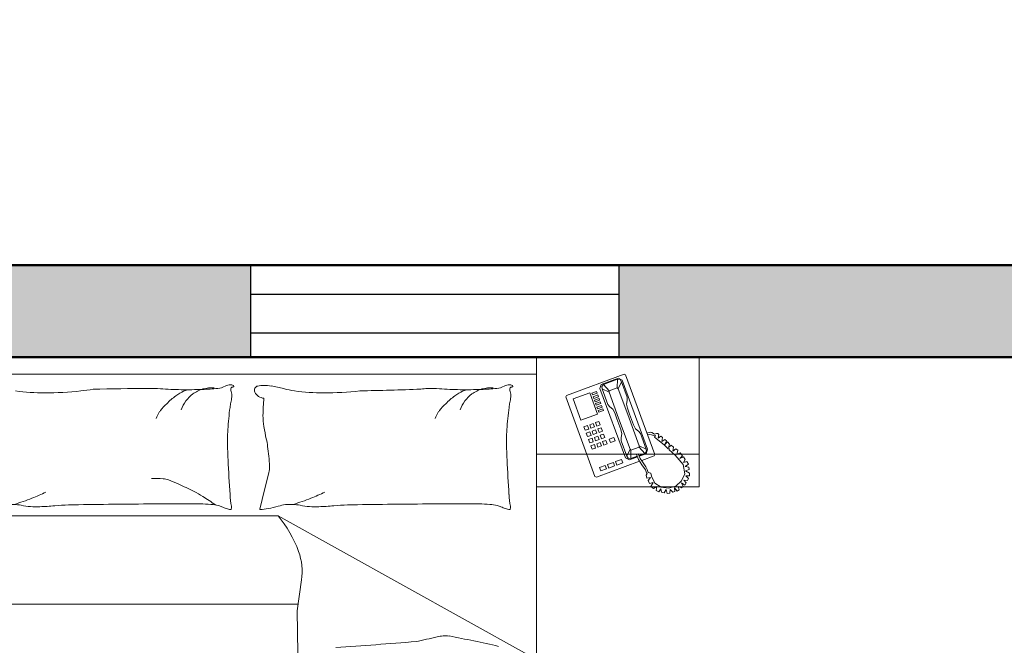
# Model space of a CAD drawing. Units: inches. Extents: x -7 to 1228, y -146 to 1091.
# Tile 55 of 88: x 96 to 193, y 964 to 1025. Entities that reach past the tile are written whole.
import ezdxf

# ---------------------------------------------------------------- set-up
doc = ezdxf.new("R2010")
doc.units = ezdxf.units.IN
for name, color, linetype, lineweight in [('A-FURN', 8, 'Continuous', 18), ('A-GLAZ', 175, 'Continuous', 25), ('A-WALL', 7, 'Continuous', 50), ('A-WALL-PATT', 251, 'Continuous', 13)]:
    doc.layers.add(name, color=color, linetype=linetype, lineweight=lineweight)
doc.styles.add('DIM_FONT', font='SIMPLEX.shx', dxfattribs={"width": 0.8})

# ---------------------------------------------------------------- blocks, each defined once
blk = doc.blocks.new('A$C4F634EDD')
for p, q in [((0.5, 2.6295), (2.3, 2.6295)), ((2.3, 2.6295), (2.3, 0.5295)), ((2.3, 2.6295), (2.8, 2.6295)), ((2.3, 2.2295), (2.3, 2.6295)), ((2.8, 2.6295), (2.8, 2.2295)), ((0.5, 2.5771), (2.3, 2.5771)), ((2.392, 2.5115), (2.5692, 2.5765)), ((2.4985, 2.5445), (2.5516, 2.564)), ((2.5062, 2.5454), (2.5487, 2.561)), ((2.5483, 2.5347), (2.5487, 2.561)), ((2.5487, 2.561), (2.5571, 2.56)), ((2.5615, 2.5536), (2.5514, 2.5318)), ((2.5516, 2.564), (2.5637, 2.5584)), ((2.5571, 2.56), (2.5615, 2.5536)), ((2.5615, 2.5536), (2.5791, 2.5058)), ((2.5637, 2.5584), (2.6418, 2.3458)), ((2.5692, 2.5765), (2.574, 2.5743)), ((2.574, 2.5743), (2.6638, 2.3298)), ((2.412, 2.5007), (2.4634, 2.5196)), ((2.4634, 2.5196), (2.4875, 2.454)), ((2.4842, 2.5232), (2.47, 2.518)), ((2.47, 2.518), (2.472, 2.5127)), ((2.472, 2.5127), (2.4862, 2.5179)), ((2.4862, 2.5179), (2.4842, 2.5232)), ((2.4946, 2.5331), (2.4985, 2.5445)), ((2.5734, 2.3187), (2.4946, 2.5331)), ((2.5062, 2.5454), (2.5004, 2.5392)), ((2.5004, 2.5392), (2.5013, 2.5315)), ((2.5013, 2.5315), (2.5188, 2.4836)), ((2.5013, 2.5315), (2.5231, 2.5214)), ((2.5235, 2.5256), (2.5062, 2.5454)), ((2.5231, 2.5214), (2.5235, 2.5256)), ((2.5523, 2.4417), (2.5231, 2.5214)), ((2.5483, 2.5347), (2.5235, 2.5256)), ((2.5514, 2.5318), (2.5483, 2.5347)), ((2.5807, 2.4521), (2.5514, 2.5318)), ((2.3898, 2.5066), (2.392, 2.5115)), ((2.4795, 2.2621), (2.3898, 2.5066)), ((2.4361, 2.4352), (2.412, 2.5007)), ((2.4881, 2.5126), (2.4739, 2.5074)), ((2.4739, 2.5074), (2.4759, 2.502)), ((2.4759, 2.502), (2.4901, 2.5073)), ((2.492, 2.5019), (2.4778, 2.4967)), ((2.4778, 2.4967), (2.4798, 2.4914)), ((2.4798, 2.4914), (2.494, 2.4966)), ((2.4959, 2.4913), (2.4817, 2.4861)), ((2.4901, 2.5073), (2.4881, 2.5126)), ((2.494, 2.4966), (2.492, 2.5019)), ((2.4979, 2.486), (2.4959, 2.4913)), ((2.5788, 2.4956), (2.5767, 2.4848)), ((2.5791, 2.5058), (2.5788, 2.4956)), ((2.4817, 2.4861), (2.4837, 2.4808)), ((2.4837, 2.4808), (2.4979, 2.486)), ((2.4998, 2.4807), (2.4856, 2.4755)), ((2.4856, 2.4755), (2.4876, 2.4702)), ((2.4876, 2.4702), (2.5018, 2.4754)), ((2.5037, 2.47), (2.4895, 2.4648)), ((2.4895, 2.4648), (2.4915, 2.4595)), ((2.4915, 2.4595), (2.5057, 2.4647)), ((2.5018, 2.4754), (2.4998, 2.4807)), ((2.5057, 2.4647), (2.5037, 2.47)), ((2.5188, 2.4836), (2.5256, 2.4761)), ((2.5256, 2.4761), (2.5342, 2.4692)), ((2.5342, 2.4692), (2.5405, 2.4574)), ((2.5405, 2.4574), (2.547, 2.4397)), ((2.5767, 2.4848), (2.5795, 2.4717)), ((2.5795, 2.4717), (2.586, 2.454)), ((2.4875, 2.454), (2.4361, 2.4352)), ((2.4811, 2.4276), (2.4917, 2.4315)), ((2.485, 2.4169), (2.4811, 2.4276)), ((2.4917, 2.4315), (2.4956, 2.4208)), ((2.5594, 2.4061), (2.547, 2.4397)), ((2.5523, 2.4417), (2.5875, 2.346)), ((2.5807, 2.4521), (2.6158, 2.3564)), ((2.5984, 2.4204), (2.586, 2.454)), ((2.4457, 2.4146), (2.4563, 2.4185)), ((2.4496, 2.4039), (2.4457, 2.4146)), ((2.4602, 2.4078), (2.4496, 2.4039)), ((2.4528, 2.3951), (2.4635, 2.399)), ((2.4563, 2.4185), (2.4602, 2.4078)), ((2.4634, 2.4211), (2.474, 2.425)), ((2.4673, 2.4104), (2.4634, 2.4211)), ((2.4635, 2.399), (2.4674, 2.3883)), ((2.4779, 2.4143), (2.4673, 2.4104)), ((2.4706, 2.4016), (2.4812, 2.4055)), ((2.4745, 2.3909), (2.4706, 2.4016)), ((2.474, 2.425), (2.4779, 2.4143)), ((2.4812, 2.4055), (2.4851, 2.3949)), ((2.4956, 2.4208), (2.485, 2.4169)), ((2.4883, 2.4081), (2.4989, 2.412)), ((2.4922, 2.3975), (2.4883, 2.4081)), ((2.5028, 2.4014), (2.4922, 2.3975)), ((2.4989, 2.412), (2.5028, 2.4014)), ((2.5622, 2.393), (2.5594, 2.4061)), ((2.6047, 2.4086), (2.5984, 2.4204)), ((2.6133, 2.4017), (2.6047, 2.4086)), ((2.6201, 2.3941), (2.6133, 2.4017)), ((2.6499, 2.3979), (2.6397, 2.3953)), ((2.6551, 2.397), (2.6499, 2.3979)), ((2.6627, 2.392), (2.6551, 2.397)), ((2.4567, 2.3844), (2.4528, 2.3951)), ((2.4674, 2.3883), (2.4567, 2.3844)), ((2.46, 2.3756), (2.4706, 2.3795)), ((2.4639, 2.365), (2.46, 2.3756)), ((2.4745, 2.3689), (2.4639, 2.365)), ((2.4706, 2.3795), (2.4745, 2.3689)), ((2.4851, 2.3949), (2.4745, 2.3909)), ((2.4777, 2.3821), (2.4883, 2.386)), ((2.4816, 2.3715), (2.4777, 2.3821)), ((2.4922, 2.3754), (2.4816, 2.3715)), ((2.4849, 2.3626), (2.4955, 2.3665)), ((2.4883, 2.386), (2.4922, 2.3754)), ((2.4954, 2.3886), (2.5061, 2.3925)), ((2.4993, 2.378), (2.4954, 2.3886)), ((2.4955, 2.3665), (2.4994, 2.3559)), ((2.51, 2.3819), (2.4993, 2.378)), ((2.5026, 2.3691), (2.5132, 2.373)), ((2.5065, 2.3585), (2.5026, 2.3691)), ((2.5061, 2.3925), (2.51, 2.3819)), ((2.5132, 2.373), (2.5171, 2.3624)), ((2.5238, 2.3769), (2.538, 2.3821)), ((2.5277, 2.3663), (2.5238, 2.3769)), ((2.5419, 2.3715), (2.5277, 2.3663)), ((2.538, 2.3821), (2.5419, 2.3715)), ((2.5598, 2.372), (2.5601, 2.3822)), ((2.5774, 2.3242), (2.5598, 2.372)), ((2.5601, 2.3822), (2.5622, 2.393)), ((2.6376, 2.3463), (2.6201, 2.3941)), ((2.6417, 2.39), (2.6488, 2.391)), ((2.6488, 2.391), (2.6538, 2.3895)), ((2.6538, 2.3895), (2.6596, 2.388)), ((2.6596, 2.388), (2.6626, 2.3867)), ((2.6626, 2.3867), (2.6662, 2.388)), ((2.6692, 2.394), (2.6627, 2.392)), ((2.6662, 2.388), (2.6632, 2.3828)), ((2.6632, 2.3828), (2.6736, 2.3744)), ((2.6736, 2.3944), (2.6692, 2.394)), ((2.6765, 2.391), (2.6736, 2.3944)), ((2.6736, 2.3744), (2.6922, 2.3593)), ((2.6742, 2.3795), (2.6765, 2.391)), ((2.6824, 2.3858), (2.6742, 2.3795)), ((2.6873, 2.3815), (2.6824, 2.3858)), ((2.6853, 2.369), (2.6873, 2.3815)), ((2.6946, 2.376), (2.6853, 2.369)), ((2.6995, 2.3713), (2.6946, 2.376)), ((2.695, 2.3603), (2.6995, 2.3713)), ((2.7031, 2.3682), (2.695, 2.3603)), ((2.7096, 2.3616), (2.7031, 2.3682)), ((2.4672, 2.3561), (2.4778, 2.36)), ((2.4711, 2.3455), (2.4672, 2.3561)), ((2.4817, 2.3494), (2.4711, 2.3455)), ((2.4778, 2.36), (2.4817, 2.3494)), ((2.4888, 2.352), (2.4849, 2.3626)), ((2.4994, 2.3559), (2.4888, 2.352)), ((2.5171, 2.3624), (2.5065, 2.3585)), ((2.5774, 2.3242), (2.5875, 2.346)), ((2.5875, 2.346), (2.5905, 2.3431)), ((2.5905, 2.3431), (2.5901, 2.3168)), ((2.6154, 2.3522), (2.5905, 2.3431)), ((2.6158, 2.3564), (2.6154, 2.3522)), ((2.6154, 2.3522), (2.6327, 2.3324)), ((2.6376, 2.3463), (2.6158, 2.3564)), ((2.6327, 2.3324), (2.6385, 2.3386)), ((2.6418, 2.3458), (2.6369, 2.332)), ((2.6385, 2.3386), (2.6376, 2.3463)), ((2.6922, 2.3593), (2.7051, 2.3473)), ((2.7051, 2.3473), (2.7079, 2.3475)), ((2.7062, 2.351), (2.7096, 2.3616)), ((2.7147, 2.3578), (2.7062, 2.351)), ((2.7079, 2.3475), (2.7079, 2.3443)), ((2.7079, 2.3443), (2.727, 2.3277)), ((2.7214, 2.3517), (2.7147, 2.3578)), ((2.7196, 2.34), (2.7214, 2.3517)), ((2.7286, 2.3466), (2.7196, 2.34)), ((2.7346, 2.3423), (2.7286, 2.3466)), ((2.732, 2.3295), (2.7346, 2.3423)), ((2.8, 2.3301), (2.3, 2.3301)), ((2.6172, 2.3086), (2.4844, 2.2599)), ((2.5362, 2.305), (2.5185, 2.2985)), ((2.5401, 2.2944), (2.5362, 2.305)), ((2.561, 2.3141), (2.5433, 2.3076)), ((2.5433, 2.3076), (2.5472, 2.297)), ((2.5649, 2.3035), (2.561, 2.3141)), ((2.5855, 2.3131), (2.5734, 2.3187)), ((2.5818, 2.3178), (2.5774, 2.3242)), ((2.5901, 2.3168), (2.5818, 2.3178)), ((2.6104, 2.3222), (2.5855, 2.3131)), ((2.5901, 2.3168), (2.6097, 2.324)), ((2.613, 2.3312), (2.6077, 2.3293)), ((2.6077, 2.3293), (2.6135, 2.3141)), ((2.6192, 2.3174), (2.613, 2.3312)), ((2.6135, 2.3141), (2.6244, 2.2977)), ((2.6153, 2.3261), (2.6327, 2.3324)), ((2.6369, 2.332), (2.6161, 2.3243)), ((2.626, 2.3069), (2.6192, 2.3174)), ((2.6616, 2.3249), (2.6234, 2.3109)), ((2.6365, 2.2916), (2.626, 2.3069)), ((2.6638, 2.3298), (2.6616, 2.3249)), ((2.727, 2.3277), (2.7512, 2.2983)), ((2.7423, 2.3345), (2.732, 2.3295)), ((2.7406, 2.3172), (2.7495, 2.325)), ((2.7519, 2.3218), (2.7406, 2.3172)), ((2.7495, 2.325), (2.7423, 2.3345)), ((2.7575, 2.3144), (2.7519, 2.3218)), ((2.7526, 2.3045), (2.7575, 2.3144)), ((2.7622, 2.308), (2.7526, 2.3045)), ((2.7673, 2.2997), (2.7622, 2.308)), ((2.5114, 2.2959), (2.4936, 2.2894)), ((2.4936, 2.2894), (2.4976, 2.2788)), ((2.4976, 2.2788), (2.5153, 2.2853)), ((2.5153, 2.2853), (2.5114, 2.2959)), ((2.5185, 2.2985), (2.5224, 2.2879)), ((2.5224, 2.2879), (2.5401, 2.2944)), ((2.5472, 2.297), (2.5649, 2.3035)), ((2.6244, 2.2977), (2.6349, 2.2825)), ((2.6349, 2.2825), (2.638, 2.273)), ((2.6407, 2.2834), (2.6365, 2.2916)), ((2.6438, 2.2739), (2.6407, 2.2834)), ((2.7512, 2.2983), (2.756, 2.2695)), ((2.7574, 2.2924), (2.7673, 2.2997)), ((2.7687, 2.2905), (2.7574, 2.2924)), ((2.7587, 2.279), (2.7699, 2.2828)), ((2.7708, 2.2725), (2.7587, 2.279)), ((2.7699, 2.2828), (2.7687, 2.2905)), ((1.4546, 2.1912), (1.4752, 2.2738)), ((2.4844, 2.2599), (2.4795, 2.2621)), ((2.6399, 2.2712), (2.6374, 2.2659)), ((2.6374, 2.2659), (2.6398, 2.257)), ((2.638, 2.273), (2.6399, 2.2712)), ((2.6398, 2.257), (2.6509, 2.259)), ((2.6509, 2.259), (2.6431, 2.2492)), ((2.6431, 2.2492), (2.6473, 2.2398)), ((2.6519, 2.2716), (2.6438, 2.2739)), ((2.6535, 2.2628), (2.6519, 2.2716)), ((2.6636, 2.2409), (2.6535, 2.2628)), ((2.7459, 2.2483), (2.7284, 2.2317)), ((2.756, 2.2695), (2.7459, 2.2483)), ((2.7529, 2.2505), (2.7645, 2.2498)), ((2.7607, 2.2424), (2.7529, 2.2505)), ((2.759, 2.2637), (2.7706, 2.2643)), ((2.7676, 2.2559), (2.759, 2.2637)), ((2.7645, 2.2498), (2.7676, 2.2559)), ((2.7706, 2.2643), (2.7708, 2.2725)), ((2.8, 2.2295), (2.3, 2.2295)), ((2.6473, 2.2398), (2.6592, 2.2429)), ((2.6592, 2.2429), (2.6521, 2.2314)), ((2.6521, 2.2314), (2.6598, 2.2248)), ((2.6598, 2.2248), (2.6697, 2.2309)), ((2.6836, 2.2287), (2.6636, 2.2409)), ((2.6697, 2.2309), (2.6684, 2.219)), ((2.6684, 2.219), (2.6761, 2.2145)), ((2.6761, 2.2145), (2.6821, 2.2237)), ((2.6821, 2.2237), (2.6843, 2.2135)), ((2.7063, 2.2256), (2.6836, 2.2287)), ((2.6927, 2.2117), (2.6986, 2.222)), ((2.6986, 2.222), (2.7019, 2.2098)), ((2.7284, 2.2317), (2.7063, 2.2256)), ((2.7102, 2.2104), (2.7113, 2.2218)), ((2.7113, 2.2218), (2.7192, 2.2137)), ((2.7192, 2.2137), (2.7255, 2.2152)), ((2.7255, 2.2152), (2.7242, 2.2265)), ((2.7242, 2.2265), (2.7324, 2.2165)), ((2.7324, 2.2165), (2.7386, 2.2208)), ((2.7386, 2.2208), (2.7354, 2.2306)), ((2.7354, 2.2306), (2.7462, 2.2264)), ((2.7509, 2.2314), (2.7459, 2.2418)), ((2.7459, 2.2418), (2.7568, 2.2352)), ((2.7462, 2.2264), (2.7509, 2.2314)), ((2.7568, 2.2352), (2.7607, 2.2424)), ((1.4471, 2.1612), (1.4546, 2.1912)), ((2.6843, 2.2135), (2.6927, 2.2117)), ((2.7019, 2.2098), (2.7102, 2.2104)), ((1.5035, 2.141), (0.5458, 2.141)), ((1.5035, 2.141), (2.2716, 1.7136)), ((1.576, 1.9433), (1.5624, 1.8479)), ((0.5458, 1.8684), (1.5653, 1.8684)), ((1.5624, 1.8479), (1.5641, 1.7178))]:
    blk.add_line(p, q)
for centre, radius, start, end in [((0.7851, 3.2019), 0.6827, 262.4531, 270), ((0.7851, 3.5682), 1.049, 270, 276.0867), ((0.8402, 3.0514), 0.5293, 276.0867, 280.1899), ((1.1602, -8.1346), 10.6675, 90.30153, 91.21582), ((1.1169, 2.2433), 0.2897, 85.1982, 92.5386), ((1.2142, 3.4021), 0.8732, 265.1982, 269.4243), ((1.2362, 2.45), 0.0768, 117.2396, 128.3886), ((1.3082, 2.3102), 0.234, 110.8603, 117.2396), ((1.2204, 4.0232), 1.4943, 269.4243, 271.9079), ((1.2995, 2.4357), 0.0992, 105.9352, 126.0864), ((1.2429, 3.3501), 0.8208, 271.9079, 275.2592), ((1.2995, 2.4357), 0.0992, 85.7841, 105.9352), ((1.3132, 2.5864), 0.0539, 275.2592, 300.6513), ((1.3554, 2.5152), 0.0289, 85.6975, 120.6513), ((1.3556, 2.519), 0.0251, 68.2117, 85.6975), ((1.3739, 2.5288), 0.0156, 158.0096, 201.421), ((1.3634, 2.533), 0.00428, 78.1069, 158.0096), ((1.3288, 2.5111), 0.0328, 351.8665, 21.421), ((1.3647, 2.5395), 0.00232, 258.1069, 19.564), ((1.3637, 2.5391), 0.00342, 19.564, 68.2117), ((1.444, 2.5274), 0.0131, 101.2724, 206.5805), ((1.4628, 2.5368), 0.0342, 206.5805, 265.5998), ((1.4591, 2.4516), 0.0904, 90, 101.2724), ((1.4591, 2.3808), 0.1611, 81.5628, 90), ((1.438, 2.2388), 0.3048, 74.256, 81.5628), ((1.5865, 2.7653), 0.2422, 254.256, 262.4531), ((1.6443, 3.2019), 0.6827, 262.4531, 270), ((1.6443, 3.5682), 1.049, 270, 276.0867), ((1.4785, 15.4878), 12.9656, 271.22425, 272.05324), ((1.97, 2.3805), 0.1524, 92.5386, 100.1899), ((1.9761, 2.2433), 0.2897, 85.1982, 92.5386), ((2.0734, 3.4021), 0.8732, 265.1982, 269.4243), ((2.0954, 2.45), 0.0768, 117.2396, 128.3886), ((2.1674, 2.3102), 0.234, 110.8603, 117.2396), ((2.0797, 4.0232), 1.4943, 269.4243, 271.9079), ((2.1588, 2.4357), 0.0992, 105.9352, 126.0864), ((2.1021, 3.3501), 0.8208, 271.9079, 275.2592), ((2.1588, 2.4357), 0.0992, 85.7841, 105.9352), ((2.1724, 2.5864), 0.0539, 275.2592, 300.6513), ((2.2146, 2.5152), 0.0289, 85.6975, 120.6513), ((2.2149, 2.519), 0.0251, 68.2117, 85.6975), ((2.2331, 2.5288), 0.0156, 158.0096, 201.421), ((2.2226, 2.533), 0.00428, 78.1069, 158.0096), ((2.1881, 2.5111), 0.0328, 351.8665, 21.421), ((2.224, 2.5395), 0.00232, 258.1069, 19.564), ((2.2229, 2.5391), 0.00342, 19.564, 68.2117), ((1.4317, 2.2032), 0.3916, 128.3886, 133.8115), ((1.2995, 2.4357), 0.0992, 143.8234, 161.5603), ((1.2995, 2.4357), 0.0992, 126.0864, 143.8234), ((1.5522, 2.448), 0.1983, 167.8905, 172.3191), ((1.1177, 2.5413), 0.246, 347.8905, 351.8665), ((1.949, 2.4496), 0.4918, 173.7676, 180), ((2.291, 2.2032), 0.3916, 128.3886, 133.8115), ((2.1588, 2.4357), 0.0992, 143.8234, 161.5603), ((2.1588, 2.4357), 0.0992, 126.0864, 143.8234), ((2.4114, 2.448), 0.1983, 167.8905, 172.3191), ((1.977, 2.5413), 0.246, 347.8905, 351.8665), ((1.3127, 2.3625), 0.2002, 151.6832, 156.9972), ((1.1799, 2.4341), 0.0493, 140.9651, 151.6832), ((1.3165, 2.3233), 0.2252, 133.8115, 140.9651), ((2.2605, 2.3525), 0.9131, 172.3191, 176.6313), ((2.1719, 2.3625), 0.2002, 151.6832, 156.9972), ((2.0391, 2.4341), 0.0493, 140.9651, 151.6832), ((2.1757, 2.3233), 0.2252, 133.8115, 140.9651), ((3.1198, 2.3525), 0.9131, 172.3191, 176.6313), ((1.6611, 2.4496), 0.204, 180, 189.6844), ((2.0266, 2.3663), 0.6787, 176.6313, 181.6331), ((2.3295, 2.5637), 0.882, 189.6844, 192.1984), ((2.8858, 2.3663), 0.6787, 176.6313, 181.6331), ((1.1575, 2.3103), 0.3171, 8.0051, 12.1984), ((2.7128, 2.3859), 1.3652, 181.6331, 183.055), ((0.8191, 2.2627), 0.6588, 2.6649, 8.0051), ((3.5721, 2.3859), 1.3652, 181.6331, 183.055), ((14.9657, 3.0398), 13.6356, 183.05496, 183.50486), ((15.8249, 3.0398), 13.6356, 183.05496, 183.50486), ((1.4096, 2.2902), 0.0677, 345.9548, 2.6649), ((1.1303, 1.9835), 0.2721, 85.9172, 93.5552), ((1.1455, 2.197), 0.058, 69.3257, 85.9172), ((0.9871, 1.7772), 0.5066, 65.6735, 69.3257), ((0.473, 2.8815), 0.7387, 293.4844, 295.3111), ((0.6058, 0.9338), 1.4323, 63.5015, 65.6735), ((1.1054, 1.9358), 0.3126, 57.865, 63.5015), ((1.3322, 2.8815), 0.7387, 293.4844, 295.3111), ((0.473, 2.8815), 0.7387, 287.1982, 289.428), ((0.473, 2.8815), 0.7387, 289.428, 291.6577), ((0.473, 2.8815), 0.7387, 291.6577, 293.4844), ((0.8841, 1.5835), 0.7286, 54.1737, 57.865), ((1.6762, 2.2258), 0.3212, 183.5049, 189.9984), ((1.3322, 2.8815), 0.7387, 287.1982, 289.428), ((1.3322, 2.8815), 0.7387, 289.428, 291.6577), ((1.3322, 2.8815), 0.7387, 291.6577, 293.4844), ((2.5355, 2.2258), 0.3212, 183.5049, 189.9984), ((0.6836, 2.0301), 0.1459, 78.4414, 96.4341), ((0.759, 2.3985), 0.2301, 258.4414, 272.7491), ((0.7026, 3.5718), 1.4048, 272.7491, 274.6176), ((0.9136, 0.9591), 1.2165, 92.6096, 94.6176), ((1.2501, -19.8405), 22.0183, 90.37908, 91.01965), ((1.2012, -3.5404), 5.7185, 89.7135, 90.9704), ((1.224, 1.0141), 1.164, 86.426, 89.7135), ((1.2875, 2.0302), 0.1459, 77.131, 86.426), ((1.3099, 2.1283), 0.0453, 62.7159, 77.131), ((1.3658, 2.2367), 0.0767, 242.7159, 253.7788), ((1.3688, 2.247), 0.0875, 253.7788, 262.8796), ((1.3581, 2.1615), 0.00132, 262.8796, 343.3022), ((1.3409, 2.1667), 0.0193, 343.3022, 9.9984), ((1.448, 2.1609), 0.000917, 165.9551, 274.0829), ((1.4288, 2.4301), 0.2708, 274.0829, 279.4841), ((1.4355, 2.3896), 0.2297, 279.4841, 287.3864), ((1.5399, 2.0561), 0.1197, 96.4341, 107.3864), ((1.5429, 2.0301), 0.1459, 78.4414, 96.4341), ((1.6182, 2.3985), 0.2301, 258.4414, 272.7491), ((1.5619, 3.5718), 1.4048, 272.7491, 274.6176), ((1.7729, 0.9591), 1.2165, 92.6096, 94.6176), ((2.1093, -19.8405), 22.0183, 90.37908, 91.01965), ((2.0605, -3.5404), 5.7185, 89.7135, 90.9704), ((2.0833, 1.0141), 1.164, 86.426, 89.7135), ((2.1467, 2.0302), 0.1459, 77.131, 86.426), ((2.1691, 2.1283), 0.0453, 62.7159, 77.131), ((2.2251, 2.2367), 0.0767, 242.7159, 253.7788), ((2.2281, 2.247), 0.0875, 253.7788, 262.8796), ((2.2174, 2.1615), 0.00132, 262.8796, 343.3022), ((2.2001, 2.1667), 0.0193, 343.3022, 9.9984), ((1.2147, 1.9017), 0.3751, 20.1488, 39.6445), ((1.3977, 1.9688), 0.1801, 351.8644, 20.1488), ((1.4194, 4.2174), 2.5158, 281.6741, 283.1904), ((2.0378, 1.5789), 0.1942, 97.7304, 103.1904), ((2.0195, 1.7137), 0.0581, 79.2724, 97.7304), ((1.2737, -2.2227), 4.0646, 77.0745, 79.2724), ((0.6102, 18.0525), 16.3521, 273.75703, 274.62393)]:
    blk.add_arc(centre, radius, start, end)
at = {"style": 'DIM_FONT', "width": 0.8, "flags": 9}
for tag, p in [('YSIZE', (0.5, 2.6295)), ('XSIZE', (0.5, 2.6295)), ('XSIZE', (2.2985, 2.6295)), ('YSIZE', (2.2985, 2.6295))]:
    blk.add_attdef(tag, p, '', height=0.0005, dxfattribs=at)
blk = doc.blocks.new('WIN-36')
for p, q in [((0, 36), (0, 0)), ((9, 36), (0, 36)), ((2.343, 36), (2.343, 0)), ((6.137, 0), (6.137, 36)), ((9, 0), (9, 36)), ((0, 0), (9, 0)), ((2.343, 0), (6.137, 0))]:
    blk.add_line(p, q)

msp = doc.modelspace()

# ---------------------------------------------------------------- hatches: boundary and pattern name
at = {"layer": 'A-WALL-PATT'}
h = msp.add_hatch(color=256, dxfattribs=at)
h.dxf.hatch_style = 1
h.paths.add_polyline_path([(69, 568), (60, 568), (60, 493), (63.289, 493), (69, 493)])
h.paths.add_polyline_path([(69, 662.405), (60, 662.405), (60, 586), (69, 586)], flags=17)
h.paths.add_polyline_path([(69, 723), (184, 723), (184, 734), (179, 734), (179, 728), (69, 728), (69, 741.623), (60, 741.623), (60, 698.405), (69, 698.405)], flags=17)
h.paths.add_polyline_path([(69, 782), (231, 782), (231, 728), (231, 723), (231, 586), (236, 586), (236, 787), (69, 787), (69, 800.126), (60, 800.126), (60, 765.623), (69, 765.623)])
h.paths.add_polyline_path([(184, 842), (189, 842), (189, 848), (173, 848), (173, 842), (179, 842), (179, 787), (184, 787)])
h.paths.add_polyline_path([(118.22, 69), (69, 69), (69, 60), (118.22, 60)])
h.paths.add_polyline_path([(227, 69), (154.22, 69), (154.22, 60), (227, 60)])
h.paths.add_polyline_path([(236, 60), (232.711, 60), (227, 60), (227, 36), (236, 36)])
h.paths.add_polyline_path([(389, 60), (380, 60), (380, 36), (389, 36)])
h.paths.add_polyline_path([(384, 181), (380, 181), (380, 115), (380, 78), (384, 78)])
h.paths.add_polyline_path([(380, 115), (334.547, 115), (334.547, 109), (380, 109)])
h.paths.add_polyline_path([(274.547, 115), (236, 115), (236, 201), (232.711, 201), (231, 201), (231, 78), (236, 78), (236, 109), (274.547, 109)])
h.paths.add_polyline_path([(69, 123), (60, 123), (60, 78), (69, 78)])
h.paths.add_polyline_path([(69, 201), (60, 201), (60, 159), (69, 159)])
h.paths.add_polyline_path([(143, 219), (69, 219), (69, 213), (143, 213)], flags=17)
h.paths.add_polyline_path([(189, 219), (184, 219), (184, 274), (231, 274), (231, 219), (236, 219), (236, 279), (184, 279), (184, 297), (179, 297), (179, 279), (69, 279), (69, 290.912), (60, 290.912), (60, 262.179), (69, 262.179), (69, 274), (179, 274), (179, 219), (173, 219), (173, 213), (189, 213)])
h.paths.add_polyline_path([(69, 238.179), (60, 238.179), (60, 219), (69, 219)], flags=17)
h.paths.add_polyline_path([(69, 333), (60, 333), (60, 314.912), (69, 314.912), (69, 316.965)])
h.paths.add_polyline_path([(190, 338), (184, 338), (69, 338), (69, 333), (179, 333), (179, 327), (184, 327), (184, 333.021), (190, 333.046)])
h.paths.add_polyline_path([(69, 386.806), (60, 386.806), (60, 351), (69, 351)])
h.paths.add_polyline_path([(69, 475), (60, 475), (60, 422.806), (69, 422.806)])
h.paths.add_polyline_path([(236, 475), (231, 475), (231, 351.238), (236, 351.238)])
h.paths.add_polyline_path([(384, 475), (380, 475), (380, 362), (384, 362)])
h.paths.add_polyline_path([(547, 307), (439, 307), (439, 356), (445, 356), (445, 362), (433, 362), (433, 307), (380, 307), (380, 244), (380, 241), (384, 241), (384, 301), (433, 301), (433, 277), (439, 277), (439, 301), (547, 301)])
h.paths.add_polyline_path([(547, 241), (439, 241), (439, 247), (433, 247), (433, 235), (547, 235)])
h.paths.add_polyline_path([(450, 69), (440.286, 69), (424.889, 69), (389, 69), (389, 60), (450, 60)])
h.paths.add_polyline_path([(547, 69), (486, 69), (486, 60), (547, 60)])
h.paths.add_polyline_path([(556, 148.268), (547, 148.268), (547, 78), (556, 78)])
h.paths.add_polyline_path([(556, 223), (547, 223), (547, 195), (547, 184.268), (556, 184.268)])
h.paths.add_polyline_path([(556, 311.192), (547, 311.192), (547, 273.075), (556, 273.075)])
h.paths.add_polyline_path([(556, 344), (552.711, 344), (547, 344), (547, 335.192), (556, 335.192)])
h.paths.add_polyline_path([(556, 249.075), (547, 249.075), (547, 241), (556, 241)])
h.paths.add_polyline_path([(547, 362), (475, 362), (475, 356), (547, 356)], flags=0)
h.paths.add_polyline_path([(556, 399.621), (547, 399.621), (547, 362), (556, 362)])
h.paths.add_polyline_path([(556, 475), (547, 475), (547, 435.621), (556, 435.621)])
h.paths.add_polyline_path([(547, 493), (389, 493), (389, 487), (547, 487)])
h.paths.add_polyline_path([(380, 493), (278, 493), (278, 487), (380, 487)])
h.paths.add_polyline_path([(227, 493), (69, 493), (69, 487), (227, 487)])
h.paths.add_polyline_path([(643, 122.445), (634, 122.445), (634, 78), (643, 78)])
h.paths.add_polyline_path([(702.5, 69), (692.786, 69), (677.389, 69), (643, 69), (643, 60), (702.5, 60)])
h.paths.add_polyline_path([(798, 69), (738.5, 69), (738.5, 60), (798, 60)])
h.paths.add_polyline_path([(807, 60), (803.711, 60), (798, 60), (798, 36), (807, 36)])
h.paths.add_polyline_path([(807, 109), (846.751, 109), (846.751, 115), (807, 115), (807, 159), (802, 159), (802, 78), (807, 78)])
h.paths.add_polyline_path([(807, 201), (802, 201), (802, 195), (807, 195)])
h.paths.add_polyline_path([(643, 201), (634, 201), (634, 158.445), (643, 158.445)])
h.paths.add_polyline_path([(756, 225), (751, 225), (751, 219), (643, 219), (643, 213), (756, 213)])
h.paths.add_polyline_path([(643, 240.848), (634, 240.848), (634, 219), (643, 219)])
h.paths.add_polyline_path([(643, 274), (643, 288.629), (634, 288.629), (634, 264.848), (643, 264.848)])
h.paths.add_polyline_path([(802, 279), (756, 279), (756, 297), (751, 297), (751, 279), (643, 279), (643, 274), (751, 274), (751, 255), (756, 255), (756, 274), (802, 274)])
h.paths.add_polyline_path([(807, 333), (803.711, 333), (802, 333), (802, 279), (802, 274), (802, 219), (807, 219)])
h.paths.add_polyline_path([(956, 182), (951, 182), (951, 115), (906.751, 115), (906.751, 109), (951, 109), (951, 78), (956, 78)])
h.paths.add_polyline_path([(960, 60), (951, 60), (951, 36), (960, 36)])
h.paths.add_polyline_path([(1021, 69), (1005.781, 69), (960, 69), (960, 60), (1021, 60)])
h.paths.add_polyline_path([(956, 224), (951, 224), (951, 218), (956, 218)])
h.paths.add_polyline_path([(956, 302), (1004, 302), (1004, 278), (1010, 278), (1010, 302), (1118, 302), (1118, 290.809), (1127, 290.809), (1127, 326.968), (1118, 326.968), (1118, 320.966), (1118, 307), (1010, 307), (1010, 356), (1016, 356), (1016, 362), (1004, 362), (1004, 307), (951, 307), (951, 244), (951, 242), (954.289, 242), (956, 242)])
h.paths.add_polyline_path([(643, 333), (634, 333), (634, 312.629), (643, 312.629), (643, 316.965)])
h.paths.add_polyline_path([(756, 338), (643, 338), (643, 333), (751, 333), (751, 327), (756, 327)])
h.paths.add_polyline_path([(643, 388), (634, 388), (634, 351), (643, 351)])
h.paths.add_polyline_path([(807, 357), (802, 357), (802, 351), (807, 351)])
h.paths.add_polyline_path([(807, 475), (802, 475), (802, 393), (807, 393)])
h.paths.add_polyline_path([(643, 475), (634, 475), (634, 424), (643, 424)])
h.paths.add_polyline_path([(798, 493), (643, 493), (643, 487), (798, 487)])
h.paths.add_polyline_path([(634, 493), (556, 493), (556, 487), (634, 487)])
h.paths.add_polyline_path([(813, 493), (807, 493), (807, 487), (813, 487)])
h.paths.add_polyline_path([(951, 493), (849, 493), (849, 487), (951, 487)])
h.paths.add_polyline_path([(956, 484), (951, 484), (951, 374), (956, 374)])
h.paths.add_polyline_path([(1109, 493), (969, 493), (969, 487), (1109, 487)])
h.paths.add_polyline_path([(1127, 484), (1118, 484), (1118, 450.641), (1127, 450.641)])
h.paths.add_polyline_path([(1127, 414.641), (1118, 414.641), (1118, 365), (1127, 365)])
h.paths.add_polyline_path([(1109, 362), (1046, 362), (1046, 356), (1109, 356)], flags=17)
h.paths.add_polyline_path([(1127, 356), (1123.454, 356), (1118, 356), (1118, 350.968), (1127, 350.968)], flags=0)
h.paths.add_polyline_path([(1127, 266.809), (1118, 266.809), (1118, 262.361), (1118, 242), (1127, 242)], flags=17)
h.paths.add_polyline_path([(1118, 242), (1010, 242), (1010, 248), (1004, 248), (1004, 237), (1118, 237)])
h.paths.add_polyline_path([(1127, 224), (1118, 224), (1118, 170), (1127, 170)])
h.paths.add_polyline_path([(1127, 134), (1118, 134), (1118, 78), (1127, 78)])
h.paths.add_polyline_path([(1118, 69), (1057, 69), (1057, 60), (1118, 60)])
h.paths.add_polyline_path([(227, 571.546), (227, 574), (69, 574), (69, 568), (227, 568)])
h.paths.add_polyline_path([(380, 571.546), (380, 574), (278, 574), (278, 568), (380, 568)])
h.paths.add_polyline_path([(242, 574), (236, 574), (236, 568), (242, 568)])
h.paths.add_polyline_path([(547, 571.546), (547, 574), (389, 574), (389, 568), (547, 568)])
h.paths.add_polyline_path([(384, 733), (380, 733), (380, 586), (384, 586)])
h.paths.add_polyline_path([(556, 646), (634, 646), (634, 655), (547, 655), (547, 586), (556, 586)])
h.paths.add_polyline_path([(634, 574), (556, 574), (556, 568), (634, 568)])
h.paths.add_polyline_path([(643, 655), (634, 655), (634, 586), (643, 586)])
h.paths.add_polyline_path([(798, 574), (643, 574), (643, 568), (798, 568)])
h.paths.add_polyline_path([(643, 663.854), (634, 663.854), (634, 655), (643, 655)])
h.paths.add_polyline_path([(556, 676.967), (547, 676.967), (547, 655), (556, 655)])
h.paths.add_polyline_path([(556, 733), (547, 733), (547, 712.967), (556, 712.967)])
h.paths.add_polyline_path([(643, 710), (634, 710), (634, 699.854), (643, 699.854)])
h.paths.add_polyline_path([(807, 668), (802, 668), (802, 586), (807, 586)])
h.paths.add_polyline_path([(951, 574), (849, 574), (849, 568), (951, 568)])
h.paths.add_polyline_path([(956, 691), (951, 691), (951, 577), (956, 577)])
h.paths.add_polyline_path([(1109, 574), (969, 574), (969, 568), (1109, 568)])
h.paths.add_polyline_path([(1127, 643.403), (1118, 643.403), (1118, 577), (1127, 577)])
h.paths.add_polyline_path([(1127, 568), (1123.454, 568), (1118, 568), (1118, 493), (1127, 493)])
h.paths.add_polyline_path([(1127, 733), (1118, 733), (1118, 679.403), (1127, 679.403)])
h.paths.add_polyline_path([(1127, 777.348), (1118, 777.348), (1118, 770.035), (1118, 751), (1127, 751)], flags=17)
h.paths.add_polyline_path([(1118, 751), (1010, 751), (1010, 757), (1004, 757), (1004, 745), (1118, 745)])
h.paths.add_polyline_path([(956, 811), (1004, 811), (1004, 787), (1010, 787), (1010, 811), (1017.874, 811), (1017.874, 811.627, -0.414214), (1018.247, 812), (1031.978, 812, -0.414214), (1032.351, 811.627), (1032.351, 811), (1118, 811), (1118, 801.348), (1127, 801.348), (1127, 834.685), (1118, 834.685), (1118, 830.238), (1118, 817), (1010, 817), (1010, 866), (1016, 866), (1016, 872), (1004, 872), (1004, 817), (956, 817), (956, 866), (951, 866), (951, 751), (954.289, 751), (956, 751)])
h.paths.add_polyline_path([(1118, 872), (1046, 872), (1046, 866), (1118, 866)], flags=17)
h.paths.add_polyline_path([(1127, 924.711), (1118, 924.711), (1118, 884), (1127, 884)])
h.paths.add_polyline_path([(1127, 866), (1123.711, 866), (1118, 866), (1118, 858.685), (1127, 858.685)], flags=17)
h.paths.add_polyline_path([(956, 983), (951, 983), (951, 952), (807, 952), (807, 983), (802, 983), (802, 902), (807, 902), (807, 946), (951, 946), (951, 884), (956, 884)])
h.paths.add_polyline_path([(807, 842), (802, 842), (802, 787), (756, 787), (756, 806), (751, 806), (751, 787), (643, 787), (643, 782), (751, 782), (751, 764), (756, 764), (756, 782), (802, 782), (802, 728), (807, 728)])
h.paths.add_polyline_path([(756, 848), (643, 848), (643, 842), (751, 842), (751, 836), (756, 836)])
h.paths.add_polyline_path([(756, 734), (751, 734), (751, 728), (643, 728), (643, 723), (756, 723)])
h.paths.add_polyline_path([(643, 749.791), (634, 749.791), (634, 728), (637.289, 728), (643, 728)])
h.paths.add_polyline_path([(643, 805.405), (634, 805.405), (634, 773.791), (643, 773.791)])
h.paths.add_polyline_path([(643, 896.663), (634, 896.663), (634, 860), (637.289, 860), (643, 860)])
h.paths.add_polyline_path([(643, 842), (634, 842), (634, 829.405), (643, 829.405)])
h.paths.add_polyline_path([(643, 983), (634, 983), (634, 932.663), (643, 932.663)])
h.paths.add_polyline_path([(1127, 983), (1118, 983), (1118, 960.711), (1127, 960.711)])
h.paths.add_polyline_path([(1118, 1001), (1077.525, 1001), (1077.525, 992), (1118, 992)])
h.paths.add_polyline_path([(1041.525, 1001), (960, 1001), (960, 992), (1041.525, 992)])
h.paths.add_polyline_path([(960, 1025), (951, 1025), (951, 1001), (954.289, 1001), (960, 1001)])
h.paths.add_polyline_path([(807, 1025), (798, 1025), (798, 1001), (807, 1001)])
h.paths.add_polyline_path([(798, 1001), (738.5, 1001), (738.5, 992), (798, 992)])
h.paths.add_polyline_path([(702.5, 1001), (643, 1001), (643, 992), (702.5, 992)])
h.paths.add_polyline_path([(547, 1001), (499.113, 1001), (499.113, 992), (547, 992)])
h.paths.add_polyline_path([(463.113, 1001), (389, 1001), (389, 992), (463.113, 992)])
h.paths.add_polyline_path([(389, 1025), (380, 1025), (380, 1022), (380, 1001), (383.289, 1001), (389, 1001)])
h.paths.add_polyline_path([(236, 1025), (227, 1025), (227, 1001), (236, 1001)])
h.paths.add_polyline_path([(236, 983), (231, 983), (231, 860), (236, 860)])
h.paths.add_polyline_path([(274.547, 952), (236, 952), (236, 946), (274.547, 946)])
h.paths.add_polyline_path([(380, 952), (334.547, 952), (334.547, 946), (380, 946)])
h.paths.add_polyline_path([(384, 983), (380, 983), (380, 884), (383.289, 884), (384, 884)])
h.paths.add_polyline_path([(227, 1001), (155.012, 1001), (155.012, 992), (162.875, 992), (227, 992)])
h.paths.add_polyline_path([(119.012, 1001), (69, 1001), (69, 992), (119.012, 992)])
h.paths.add_polyline_path([(69, 983), (60, 983), (60, 922.987), (69, 922.987)])
h.paths.add_polyline_path([(69, 886.987), (60, 886.987), (60, 860), (63.289, 860), (69, 860)])
h.paths.add_polyline_path([(143, 848), (69, 848), (69, 842), (143, 842)])

# ---------------------------------------------------------------- linework, layer by layer
at = {"layer": 'A-WALL'}
for p, q in [((236, 1001), (60, 1001)), ((231, 992), (69, 992))]:
    msp.add_line(p, q, dxfattribs=at)

# ---------------------------------------------------------------- block references
at = {"layer": 'A-FURN', "xscale": 31.78426361944092, "yscale": 31.78426361944092, "zscale": 31.78426361944092}
msp.add_blockref('A$C4F634EDD', (73.879, 908.423), dxfattribs=at)
at = {"layer": 'A-GLAZ', "extrusion": (0, 0, -1), "zscale": -1, "rotation": 90.00000000000003}
msp.add_blockref('WIN-36', (-119.012, 992), dxfattribs=at)

doc.saveas('drawing.dxf')
